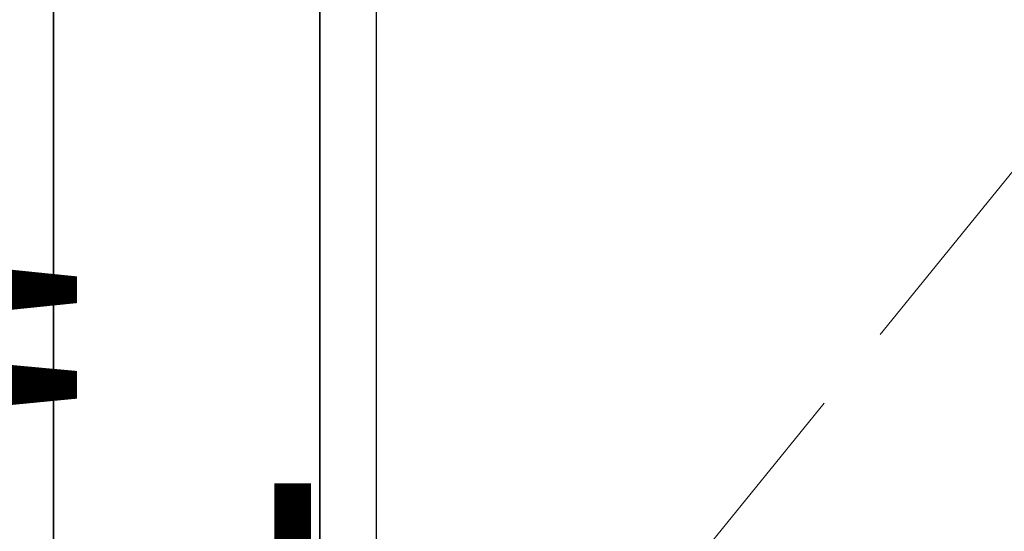
# Model space of a CAD drawing. Units: inches. Extents: x 2083 to 3317, y 1141 to 2115.
# Tile 78 of 256: x 2226 to 2259, y 1494 to 1512. Entities that reach past the tile are written whole.
import ezdxf

# ---------------------------------------------------------------- set-up
doc = ezdxf.new("R2010")
doc.units = ezdxf.units.IN
doc.linetypes.add('ACAD_ISO02W100', pattern=[15, 12, -3])
for name, color, linetype, lineweight in [('A-ANNO-DIMS', 2, 'Continuous', 18), ('A-FLOR-OPEN', 8, 'ACAD_ISO02W100', 13), ('A-WALL', 7, 'Continuous', 35)]:
    doc.layers.add(name, color=color, linetype=linetype, lineweight=lineweight)
doc.layers.add('A-WALL-PATT', color=251, linetype='Continuous', lineweight=13, true_color=0x636466)
doc.styles.get("Standard").update_dxf_attribs({"font": 'arial.ttf'})
doc.dimstyles.new('ISO-25', dxfattribs={"dimtxt": 12, "dimasz": 12, "dimexe": 1.25, "dimexo": 0.625, "dimtad": 1, "dimlunit": 3, "dimtxsty": 'Standard', "dimcen": 2.5, "dimadec": 0, "dimazin": 0, "dimtfac": 1, "dimtmove": 0, "dimatfit": 3, "dimfxl": 1, "dimarcsym": 0})

# ---------------------------------------------------------------- blocks, each defined once
blk = doc.blocks.new('*D31')
at = {"layer": 'A-ANNO-DIMS', "color": 0, "lineweight": -2, "transparency": 16777216}
for p, q in [((2237.871, 1456.649), (2237.871, 1541.915)), ((2239.393, 1444.649), (2236.621, 1444.649)), ((2237.871, 1431.548), (2237.871, 1444.649)), ((2239.393, 1431.548), (2236.621, 1431.548)), ((2237.871, 1419.548), (2237.871, 1407.548))]:
    blk.add_line(p, q, dxfattribs=at)
at = {"layer": 'A-ANNO-DIMS', "color": 0, "transparency": 16777216}
for points in [[(2235.871, 1456.649), (2239.871, 1456.649), (2237.871, 1444.649)], [(2235.871, 1419.548), (2239.871, 1419.548), (2237.871, 1431.548)]]:
    blk.add_solid(points, dxfattribs=at)
at = {"layer": 'Defpoints', "color": 0, "transparency": 16777216}
for p in [(2237.871, 1444.649), (2240.018, 1444.649), (2240.018, 1431.548)]:
    blk.add_point(p, dxfattribs=at)
at = {"layer": 'A-ANNO-DIMS', "color": 0, "transparency": 16777216, "insert": (2231.217, 1505.282), "char_height": 12, "attachment_point": 5, "rotation": 90}
blk.add_mtext('1\'-1" TYP.', dxfattribs=at)
blk = doc.blocks.new('*D45')
at = {"layer": 'A-ANNO-DIMS', "color": 0, "lineweight": -2, "transparency": 16777216}
for p, q in [((2235.96, 1478.386), (2235.96, 1531.361)), ((2418.96, 1478.386), (2418.96, 1531.361)), ((2247.96, 1530.111), (2406.96, 1530.111))]:
    blk.add_line(p, q, dxfattribs=at)
at = {"layer": 'A-ANNO-DIMS', "color": 0, "transparency": 16777216}
for points in [[(2247.96, 1532.111), (2247.96, 1528.111), (2235.96, 1530.111)], [(2406.96, 1532.111), (2406.96, 1528.111), (2418.96, 1530.111)]]:
    blk.add_solid(points, dxfattribs=at)
at = {"layer": 'Defpoints', "color": 0, "transparency": 16777216}
for p in [(2418.96, 1530.111), (2235.96, 1477.761), (2418.96, 1477.761)]:
    blk.add_point(p, dxfattribs=at)
at = {"layer": 'A-ANNO-DIMS', "color": 0, "transparency": 16777216, "insert": (2327.46, 1536.867), "char_height": 12, "attachment_point": 5}
blk.add_mtext('15\'-3"', dxfattribs=at)
blk = doc.blocks.new('*D62')
at = {"layer": 'A-ANNO-DIMS', "color": 0, "lineweight": -2, "transparency": 16777216}
for p, q in [((2235.96, 1469.386), (2235.96, 1522.361)), ((2379.96, 1469.386), (2379.96, 1522.361)), ((2247.96, 1521.111), (2367.96, 1521.111))]:
    blk.add_line(p, q, dxfattribs=at)
at = {"layer": 'A-ANNO-DIMS', "color": 0, "transparency": 16777216}
for points in [[(2247.96, 1523.111), (2247.96, 1519.111), (2235.96, 1521.111)], [(2367.96, 1523.111), (2367.96, 1519.111), (2379.96, 1521.111)]]:
    blk.add_solid(points, dxfattribs=at)
at = {"layer": 'Defpoints', "color": 0, "transparency": 16777216}
for p in [(2379.96, 1521.111), (2235.96, 1468.761), (2379.96, 1468.761)]:
    blk.add_point(p, dxfattribs=at)
at = {"layer": 'A-ANNO-DIMS', "color": 0, "transparency": 16777216, "insert": (2307.96, 1527.863), "char_height": 12, "attachment_point": 5}
blk.add_mtext('12\'-0"', dxfattribs=at)
blk = doc.blocks.new('*D64')
at = {"layer": 'A-ANNO-DIMS', "color": 0, "lineweight": -2, "transparency": 16777216}
for p, q in [((2236.585, 1702.761), (2289.56, 1702.761)), ((2288.31, 1690.761), (2288.31, 1489.761)), ((2236.585, 1477.761), (2289.56, 1477.761))]:
    blk.add_line(p, q, dxfattribs=at)
at = {"layer": 'A-ANNO-DIMS', "color": 0, "transparency": 16777216}
for points in [[(2286.31, 1690.761), (2290.31, 1690.761), (2288.31, 1702.761)], [(2286.31, 1489.761), (2290.31, 1489.761), (2288.31, 1477.761)]]:
    blk.add_solid(points, dxfattribs=at)
at = {"layer": 'Defpoints', "color": 0, "transparency": 16777216}
for p in [(2235.96, 1702.761), (2235.96, 1477.761), (2288.31, 1477.761)]:
    blk.add_point(p, dxfattribs=at)
at = {"layer": 'A-ANNO-DIMS', "color": 0, "transparency": 16777216, "insert": (2281.558, 1590.261), "char_height": 12, "attachment_point": 5, "rotation": 90}
blk.add_mtext('18\'-9"', dxfattribs=at)

msp = doc.modelspace()

# ---------------------------------------------------------------- hatches: boundary and pattern name
at = {"layer": 'A-WALL-PATT'}
h = msp.add_hatch(color=256, dxfattribs=at)
h.dxf.hatch_style = 1
h.paths.add_polyline_path([(3126.96, 2020.761), (2748.96, 2020.761), (2604.96, 2020.761), (2226.96, 2020.761), (2226.96, 1702.761), (2466.96, 1702.761), (2466.96, 1582.761), (2418.96, 1582.761), (2418.96, 1477.761), (2226.96, 1477.761), (2226.96, 1263.261), (2544.96, 1263.261), (2544.96, 1411.761), (2604.96, 1411.761), (2685.96, 1411.761), (2685.96, 1420.761), (2604.96, 1420.761), (2604.96, 1573.761), (2604.96, 1702.761), (2604.96, 2011.761), (2748.96, 2011.761), (2748.96, 1702.761), (2862.96, 1702.761), (2862.96, 1621.761), (2871.96, 1621.761), (2871.96, 1702.761), (2883.96, 1702.761), (2883.96, 1706.939, -0.026459), (2883.96, 1711.761), (2757.96, 1711.761), (2757.96, 1807.761), (2787.96, 1807.761), (2787.96, 1812.261), (2757.96, 1812.261), (2757.96, 2011.761), (2877.96, 2011.761), (2877.96, 1812.261), (2847.96, 1812.261), (2847.96, 1807.761), (2889.836, 1807.761), (2889.836, 1812.261), (2882.46, 1812.261), (2882.46, 2011.761), (3117.96, 2011.761), (3117.96, 1812.261), (2937.836, 1812.261), (2937.836, 1807.761), (2995.71, 1807.761), (2995.71, 1796.118), (3000.21, 1796.118), (3000.21, 1807.761), (3117.96, 1807.761), (3117.96, 1711.761), (3000.21, 1711.761), (3000.21, 1760.118), (2998.573, 1760.118, -0.020711), (2995.71, 1760.118), (2995.71, 1711.761), (2931.96, 1711.761), (2931.96, 1702.761), (3126.96, 1702.761)])
h.paths.add_polyline_path([(2471.46, 2011.761), (2471.46, 1810.011), (2462.717, 1810.011), (2462.717, 1805.511), (2505.96, 1805.511), (2505.96, 1810.011), (2475.96, 1810.011), (2475.96, 2011.761), (2595.96, 2011.761), (2595.96, 1810.011), (2565.96, 1810.011), (2565.96, 1805.511), (2595.96, 1805.511), (2595.96, 1711.761), (2235.96, 1711.761), (2235.96, 1805.511), (2353.71, 1805.511), (2353.71, 1796.054), (2358.21, 1796.054), (2358.21, 1805.511), (2414.717, 1805.511), (2414.717, 1810.011), (2235.96, 1810.011), (2235.96, 2011.761)], flags=16)
h.paths.add_polyline_path([(2270.205, 1994.61), (2270.205, 1970.61), (2246.205, 1970.61), (2246.205, 1994.61)], flags=0)
edge = h.paths.add_edge_path(flags=0)
edge.add_ellipse((2332.027, 1899.798), major_axis=(-3.043, 3.043), ratio=0.168252, start_angle=-161.3322, end_angle=-156.3071, ccw=False)
edge.add_ellipse((2333.082, 1898.744), major_axis=(-1.055, 1.055), ratio=0.453532, start_angle=-123.371, end_angle=-94.1591)
edge = h.paths.add_edge_path(flags=0)
edge.add_ellipse((2332.027, 1968.876), major_axis=(3.043, 3.043), ratio=0.168252, start_angle=18.6678, end_angle=23.6929)
edge.add_spline(control_points=[(2332.926, 1970.691), (2332.227, 1970.336), (2330.894, 1969.659), (2328.413, 1970.932), (2327.204, 1967.749), (2324.71, 1969.956), (2322.533, 1967.012), (2320.013, 1971.296), (2317.68, 1968.158), (2316.041, 1967.102), (2315.427, 1966.81)], knot_values=[0, 0, 0, 0, 2.267059, 4.324559, 6.685584, 8.878641, 11.121502, 14.300359, 17.755284, 19.732645, 19.732645, 19.732645, 19.732645], degree=3, periodic=0)
edge.add_ellipse((2332.027, 1968.876), major_axis=(3.043, 3.043), ratio=0.168252, start_angle=18.6678, end_angle=23.6929, ccw=False)
edge.add_ellipse((2333.082, 1969.931), major_axis=(1.055, 1.055), ratio=0.453532, start_angle=56.629, end_angle=85.8409, ccw=False)
edge = h.paths.add_edge_path(flags=0)
edge.add_spline(control_points=[(2296.428, 1967.988), (2293.628, 1965.336), (2287.704, 1959.727), (2299.744, 1949.996), (2294.533, 1935.669), (2290.573, 1920.604), (2293.394, 1909.974), (2296.185, 1904.967)], knot_values=[0.099185, 0.099185, 0.099185, 0.099185, 0.345301, 0.619822, 0.982653, 1.386093, 1.810555, 1.810555, 1.810555, 1.810555], degree=3, periodic=0)
edge.add_spline(control_points=[(2296.185, 1904.967), (2297.384, 1902.619), (2298.001, 1901.949), (2298.553, 1901.468)], knot_values=[0.006246, 0.006246, 0.006246, 0.006246, 0.055476, 0.055476, 0.055476, 0.055476], degree=3, periodic=0)
edge.add_spline(control_points=[(2298.553, 1901.468), (2297.259, 1900.923), (2295.225, 1900.232), (2293.06, 1900.614), (2292.101, 1900.788), (2292.09, 1900.791)], knot_values=[0.312835, 0.312835, 0.312835, 0.312835, 0.40178, 0.474987, 0.475903, 0.475903, 0.475903, 0.475903], degree=3, periodic=0)
edge.add_arc((2292.794, 1904.664), 3.937, 215.4209, 259.6982, ccw=False)
edge.add_spline(control_points=[(2289.585, 1902.382), (2289.477, 1902.535), (2289.368, 1902.688), (2289.261, 1902.841)], knot_values=[0.102872, 0.102872, 0.102872, 0.102872, 0.116896, 0.116896, 0.116896, 0.116896], degree=3, periodic=0)
edge.add_spline(control_points=[(2289.261, 1902.841), (2288.687, 1902.55), (2287.64, 1902.02), (2285.881, 1901.874), (2283.853, 1901.504), (2281.72, 1899.711), (2278.467, 1899.493), (2276.157, 1901.883), (2272.259, 1899.804), (2267.778, 1901.843), (2262.244, 1900.184), (2257.415, 1901.782), (2254.318, 1900.726), (2253.178, 1900.337)], knot_values=[0, 0, 0, 0, 1.907977, 3.477176, 5.261074, 7.972851, 11.680248, 13.717921, 16.939592, 22.789562, 27.502503, 33.595215, 37.145618, 37.145618, 37.145618, 37.145618], degree=3, periodic=0)
edge.add_line((2253.178, 1900.337), (2250.244, 1902.841))
edge.add_line((2250.244, 1902.841), (2250.244, 1965.833))
edge.add_line((2250.244, 1965.833), (2253.178, 1968.337))
edge.add_spline(control_points=[(2253.178, 1968.337), (2254.318, 1967.948), (2257.415, 1966.892), (2262.244, 1968.49), (2267.778, 1966.831), (2271.527, 1968.537), (2273.876, 1967.828), (2274.207, 1967.728)], knot_values=[0, 0, 0, 0, 0.09018, 0.244935, 0.364644, 0.513233, 0.537855, 0.537855, 0.537855, 0.537855], degree=3, periodic=0)
edge.add_arc((2274.353, 1963.793), 3.937, 72.0511, 92.1279, ccw=False)
edge.add_arc((2281.297, 1985.23), 18.596, 252.0511, 288.5657)
edge.add_arc((2292.317, 1956.029), 12.646, 71.0268, 113.7782, ccw=False)
edge = h.paths.add_edge_path(flags=0)
edge.add_spline(control_points=[(2274.899, 1951.856), (2275.066, 1951.617), (2275.233, 1951.377), (2275.398, 1951.136)], knot_values=[1.409916, 1.409916, 1.409916, 1.409916, 1.43159, 1.43159, 1.43159, 1.43159], degree=3, periodic=0)
edge.add_spline(control_points=[(2275.398, 1951.136), (2275.792, 1950.562), (2276.179, 1949.984), (2276.546, 1949.397)], knot_values=[1.358238, 1.358238, 1.358238, 1.358238, 1.409916, 1.409916, 1.409916, 1.409916], degree=3, periodic=0)
edge.add_line((2276.546, 1949.397), (2277.437, 1947.862))
edge.add_spline(control_points=[(2277.437, 1947.862), (2276.304, 1945.673), (2274.64, 1942.427), (2274.632, 1938.094), (2272.799, 1930.852), (2274.356, 1943.897), (2275.948, 1947.923), (2276.546, 1949.397)], knot_values=[0.005632, 0.005632, 0.005632, 0.005632, 0.186014, 0.266002, 0.357087, 0.59639, 0.739732, 0.739732, 0.739732, 0.739732], degree=3, periodic=0)
edge.add_spline(control_points=[(2276.546, 1949.397), (2276.179, 1949.984), (2275.792, 1950.562), (2275.398, 1951.136)], knot_values=[1.358238, 1.358238, 1.358238, 1.358238, 1.409916, 1.409916, 1.409916, 1.409916], degree=3, periodic=0)
edge.add_spline(control_points=[(2275.398, 1951.136), (2274.943, 1950.08), (2274.208, 1948.025), (2273.935, 1944.851), (2272.469, 1937.627), (2273.466, 1945.696), (2274.701, 1951.059), (2274.899, 1951.856)], knot_values=[0.104364, 0.104364, 0.104364, 0.104364, 0.189636, 0.269624, 0.36071, 0.600013, 0.644622, 0.644622, 0.644622, 0.644622], degree=3, periodic=0)
h.paths.add_polyline_path([(2269.168, 1963.128, -0.357527), (2268.171, 1960.976, -0.092561), (2268.171, 1939.436, -0.357527), (2269.168, 1937.285, -0.357527), (2267.016, 1938.282, -0.164785), (2254.686, 1938.282, -0.357527), (2252.534, 1937.285, -0.357527), (2253.531, 1939.436, -0.092561), (2253.531, 1960.976, -0.357527), (2252.534, 1963.128, -0.357527), (2254.686, 1962.131, -0.164785), (2267.016, 1962.131, -0.357527)], flags=0)
h.paths.add_polyline_path([(2248.874, 1967.802), (2248.874, 1957.028), (2249.458, 1957.028), (2249.458, 1911.647), (2248.874, 1911.647), (2248.874, 1900.873), (2246.512, 1900.873, 0.197327), (2244.15, 1902.457), (2244.15, 1966.218, 0.197327), (2246.512, 1967.802)], flags=0)
h.paths.add_polyline_path([(2269.168, 1931.389, -0.357527), (2268.171, 1929.238, -0.092561), (2268.171, 1907.698, -0.357527), (2269.168, 1905.547, -0.357527), (2267.016, 1906.544, -0.164785), (2254.686, 1906.544, -0.357527), (2252.534, 1905.547, -0.357527), (2253.531, 1907.698, -0.092561), (2253.531, 1929.238, -0.357527), (2252.534, 1931.389, -0.357527), (2254.686, 1930.392, -0.164785), (2267.016, 1930.392, -0.357527)], flags=0)
edge = h.paths.add_edge_path(flags=0)
edge.add_spline(control_points=[(2276.197, 1906.724), (2276.168, 1909.029), (2276.114, 1913.372), (2270.598, 1924.925), (2273.905, 1919.013), (2275.922, 1916.262), (2275.475, 1912.402), (2277.258, 1910.381), (2276.696, 1908.225), (2276.646, 1906.813), (2276.618, 1906.008)], knot_values=[0, 0, 0, 0, 8.61026, 16.221274, 18.843057, 23.804898, 27.440828, 29.356102, 31.203478, 33.650687, 33.650687, 33.650687, 33.650687], degree=3, periodic=0)
edge.add_spline(control_points=[(2276.618, 1906.008), (2276.623, 1905.624), (2276.498, 1904.629), (2275.442, 1903.855), (2274.937, 1903.08), (2274.859, 1902.841)], knot_values=[0.156488, 0.156488, 0.156488, 0.156488, 0.184398, 0.231376, 0.250598, 0.250598, 0.250598, 0.250598], degree=3, periodic=0)
edge.add_line((2274.859, 1902.841), (2276.506, 1902.841))
edge.add_spline(control_points=[(2276.506, 1902.841), (2276.788, 1903.085), (2277.665, 1904.125), (2278.25, 1904.341), (2277.654, 1908.527), (2278.156, 1906.228), (2278.1, 1905.286), (2278.847, 1904.069), (2277.857, 1903.415), (2277.874, 1902.991), (2277.904, 1902.841)], knot_values=[0.059574, 0.059574, 0.059574, 0.059574, 0.080753, 0.103741, 0.16972, 0.176036, 0.207137, 0.240474, 0.262341, 0.27366, 0.27366, 0.27366, 0.27366], degree=3, periodic=0)
edge.add_line((2277.904, 1902.841), (2280.03, 1902.841))
edge.add_spline(control_points=[(2280.03, 1902.841), (2279.888, 1903.088), (2279.499, 1903.982), (2280.152, 1905.939), (2278.104, 1909.658), (2279.762, 1907.185), (2280.328, 1904.875), (2280.485, 1903.49), (2281.463, 1903.249), (2281.758, 1902.936), (2281.834, 1902.841)], knot_values=[0.013856, 0.013856, 0.013856, 0.013856, 0.034874, 0.088867, 0.107879, 0.126738, 0.158714, 0.193757, 0.217487, 0.226722, 0.226722, 0.226722, 0.226722], degree=3, periodic=0)
edge.add_spline(control_points=[(2281.834, 1902.841), (2281.788, 1902.827), (2281.647, 1902.783), (2281.396, 1902.859), (2281.088, 1902.985), (2280.721, 1903.061), (2280.333, 1903.026), (2280.125, 1902.899), (2280.03, 1902.841)], knot_values=[0, 0, 0, 0, 0.14413, 0.435517, 0.749276, 1.153046, 1.548371, 1.878348, 1.878348, 1.878348, 1.878348], degree=3, periodic=0)
edge.add_line((2280.03, 1902.841), (2277.904, 1902.841))
edge.add_spline(control_points=[(2277.904, 1902.841), (2277.893, 1902.796), (2277.865, 1902.68), (2277.607, 1902.687), (2277.274, 1902.801), (2276.838, 1902.62), (2276.584, 1902.789), (2276.506, 1902.841)], knot_values=[0, 0, 0, 0, 0.127189, 0.326199, 0.628009, 1.24357, 1.515331, 1.515331, 1.515331, 1.515331], degree=3, periodic=0)
edge.add_line((2276.506, 1902.841), (2274.859, 1902.841))
edge.add_spline(control_points=[(2274.859, 1902.841), (2274.814, 1902.899), (2274.725, 1903.013), (2274.493, 1903.119), (2274.244, 1902.961), (2273.937, 1903.185), (2273.614, 1902.983), (2273.408, 1902.883), (2273.322, 1902.841)], knot_values=[0, 0, 0, 0, 0.21843, 0.436957, 0.687977, 0.990379, 1.398396, 1.69185, 1.69185, 1.69185, 1.69185], degree=3, periodic=0)
edge.add_spline(control_points=[(2273.322, 1902.841), (2273.617, 1903.446), (2274.274, 1904.538), (2276.027, 1904.574), (2276.207, 1906.584), (2276.197, 1906.724)], knot_values=[0.012227, 0.012227, 0.012227, 0.012227, 0.059472, 0.106218, 0.134458, 0.134458, 0.134458, 0.134458], degree=3, periodic=0)
h.paths.add_polyline_path([(2270.776, 1897.79), (2270.776, 1873.79), (2246.776, 1873.79), (2246.776, 1897.79)], flags=0)
h.paths.add_polyline_path([(2353.71, 1760.005), (2353.71, 1760.054), (2358.21, 1760.054, -0.033729)], flags=0)
h.paths.add_polyline_path([(2321.819, 1737.529), (2341.995, 1737.529, -0.414214), (2343.203, 1736.321), (2343.203, 1721.021, -0.414214), (2341.995, 1719.813), (2321.819, 1719.813, -0.414214), (2320.611, 1721.021), (2320.611, 1736.321, -0.414214)], flags=0)
h.paths.add_polyline_path([(2324.235, 1736.321), (2339.579, 1736.321, -0.414214), (2341.995, 1733.905), (2341.995, 1725.45, -0.414214), (2339.579, 1723.034), (2333.681, 1723.034), (2333.845, 1722.045, -0.870646), (2335.425, 1721.826, -0.767327), (2333.923, 1721.423), (2331.291, 1721.423, -0.767327), (2329.788, 1721.826, -0.870646), (2331.368, 1722.045), (2331.533, 1723.034), (2324.235, 1723.034, -0.414214), (2321.819, 1725.45), (2321.819, 1733.905, -0.414214)], flags=0)
h.paths.add_polyline_path([(2570.484, 1928.615), (2589.684, 1928.615), (2590.169, 1928.615), (2590.169, 1904.993), (2570.484, 1904.993)], flags=0)
h.paths.add_polyline_path([(2574.447, 1927.264, -1), (2572.829, 1927.264, -1)], flags=0)
h.paths.add_polyline_path([(2573.09, 1926.941), (2573.925, 1927.776), (2574.148, 1927.553), (2573.313, 1926.718)], flags=0)
h.paths.add_polyline_path([(2578.779, 1919.73, -1), (2571.592, 1919.73, -1)], flags=0)
h.paths.add_polyline_path([(2578.385, 1919.73, -1), (2571.985, 1919.73, -1)], flags=0)
h.paths.add_polyline_path([(2331.596, 1729.476, -1), (2333.618, 1729.476, -1)], flags=0)
h.paths.add_polyline_path([(2578.034, 1927.264, -1), (2576.416, 1927.264, -1)], flags=0)
h.paths.add_polyline_path([(2576.689, 1927.531), (2576.912, 1927.754), (2577.747, 1926.919), (2577.524, 1926.696)], flags=0)
h.paths.add_polyline_path([(2578.139, 1909.86, -1), (2572.232, 1909.86, -1)], flags=0)
h.paths.add_polyline_path([(2577.745, 1909.86, -1), (2572.625, 1909.86, -1)], flags=0)
h.paths.add_polyline_path([(2583.798, 1927.264, -1), (2582.179, 1927.264, -1)], flags=0)
h.paths.add_polyline_path([(2582.719, 1927.754), (2583.554, 1926.919), (2583.331, 1926.696), (2582.496, 1927.531)], flags=0)
h.paths.add_polyline_path([(2582.496, 1927.531), (2582.719, 1927.754), (2583.554, 1926.919), (2583.331, 1926.696)], flags=0)
h.paths.add_polyline_path([(2587.739, 1920.53, -1), (2581.832, 1920.53, -1)], flags=0)
h.paths.add_polyline_path([(2587.345, 1920.53, -1), (2582.225, 1920.53, -1)], flags=0)
h.paths.add_polyline_path([(2587.385, 1927.264, -1), (2585.766, 1927.264, -1)], flags=0)
h.paths.add_polyline_path([(2586.082, 1926.98), (2586.917, 1927.815), (2587.14, 1927.593), (2586.305, 1926.758)], flags=0)
h.paths.add_polyline_path([(2588.379, 1910.66, -1), (2581.192, 1910.66, -1)], flags=0)
h.paths.add_polyline_path([(2587.985, 1910.66, -1), (2581.585, 1910.66, -1)], flags=0)
h.paths.add_polyline_path([(2417.168, 1729.478), (2437.344, 1729.478, -0.414214), (2438.552, 1728.27), (2438.552, 1712.969, -0.414214), (2437.344, 1711.761), (2417.168, 1711.761, -0.414214), (2415.96, 1712.969), (2415.96, 1728.27, -0.414214)], flags=0)
h.paths.add_polyline_path([(2419.584, 1728.27), (2434.928, 1728.27, -0.414214), (2437.344, 1725.854), (2437.344, 1717.398, -0.414214), (2434.928, 1714.983), (2429.029, 1714.983), (2429.194, 1713.994, -0.870646), (2430.774, 1713.775, -0.767327), (2429.271, 1713.372), (2426.64, 1713.372, -0.767327), (2425.137, 1713.775, -0.870646), (2426.717, 1713.994), (2426.882, 1714.983), (2419.584, 1714.983, -0.414214), (2417.168, 1717.398), (2417.168, 1725.854, -0.414214)], flags=0)
h.paths.add_polyline_path([(2419.584, 1728.27), (2434.928, 1728.27, -0.414214), (2437.344, 1725.854), (2437.344, 1717.398, -0.414214), (2434.928, 1714.983), (2429.029, 1714.983), (2428.358, 1719.009), (2427.553, 1719.009), (2426.882, 1714.983), (2419.584, 1714.983, -0.414214), (2417.168, 1717.398), (2417.168, 1725.854, -0.414214)], flags=0)
h.paths.add_polyline_path([(2426.944, 1721.425, -1), (2428.967, 1721.425, -1)], flags=0)
h.paths.add_polyline_path([(2475.96, 1702.761), (2595.96, 1702.761), (2595.96, 1582.761), (2475.96, 1582.761)], flags=16)
h.paths.add_polyline_path([(2427.96, 1573.761), (2595.96, 1573.761), (2595.96, 1468.761), (2595.96, 1420.761), (2384.46, 1420.761), (2384.46, 1468.761), (2427.96, 1468.761)], flags=16)
h.paths.add_polyline_path([(2379.96, 1468.761), (2379.96, 1420.761), (2235.96, 1420.761), (2235.96, 1468.761)], flags=16)
h.paths.add_polyline_path([(2317.816, 1466.696), (2337.992, 1466.696, -0.414214), (2339.2, 1465.488), (2339.2, 1450.187, -0.414214), (2337.992, 1448.979), (2317.816, 1448.979, -0.414214), (2316.608, 1450.187), (2316.608, 1465.488, -0.414214)], flags=0)
h.paths.add_polyline_path([(2320.232, 1465.488), (2335.576, 1465.488, -0.414214), (2337.992, 1463.072), (2337.992, 1454.616, -0.414214), (2335.576, 1452.2), (2329.677, 1452.2), (2329.842, 1451.212, -0.870646), (2331.422, 1450.992, -0.767327), (2329.92, 1450.59), (2327.288, 1450.59, -0.767327), (2325.785, 1450.992, -0.870646), (2327.365, 1451.212), (2327.53, 1452.2), (2320.232, 1452.2, -0.414214), (2317.816, 1454.616), (2317.816, 1463.072, -0.414214)], flags=0)
h.paths.add_polyline_path([(2320.232, 1465.488), (2335.576, 1465.488, -0.414214), (2337.992, 1463.072), (2337.992, 1454.616, -0.414214), (2335.576, 1452.2), (2329.677, 1452.2), (2329.006, 1456.227), (2328.201, 1456.227), (2327.53, 1452.2), (2320.232, 1452.2, -0.414214), (2317.816, 1454.616), (2317.816, 1463.072, -0.414214)], flags=0)
h.paths.add_polyline_path([(2327.593, 1458.643, -1), (2329.615, 1458.643, -1)], flags=0)
h.paths.add_polyline_path([(2244.412, 1433.34), (2241.921, 1433.34, -0.414214), (2240.018, 1435.244), (2240.018, 1440.953, -0.414211), (2241.921, 1442.856), (2244.412, 1442.856, -1.976472)], flags=0)
h.paths.add_polyline_path([(2245.357, 1434.398, -0.414214), (2245.357, 1441.799, -2.144098)], flags=0)
h.paths.add_polyline_path([(2535.96, 1416.261), (2535.96, 1272.261), (2235.96, 1272.261), (2235.96, 1416.261)], flags=16)
h.paths.add_polyline_path([(2260.12, 1384.293), (2260.12, 1362.039), (2237.865, 1362.039), (2237.865, 1384.293)], flags=0)
edge = h.paths.add_edge_path(flags=0)
edge.add_line((2318.252, 1362.093), (2318.146, 1362.001))
edge.add_ellipse((2317.445, 1360.431), major_axis=(2.822, 2.822), ratio=0.168252, start_angle=18.6678, end_angle=20.9481, ccw=False)
edge.add_ellipse((2318.423, 1361.409), major_axis=(0.978, 0.978), ratio=0.453532, start_angle=56.629, end_angle=70.2262, ccw=False)
edge = h.paths.add_edge_path(flags=0)
edge.add_line((2319.107, 1295.571), (2319.015, 1295.677))
edge.add_ellipse((2317.445, 1296.378), major_axis=(-2.822, 2.822), ratio=0.168252, start_angle=-161.3322, end_angle=-159.0519, ccw=False)
edge.add_ellipse((2318.423, 1295.4), major_axis=(-0.978, 0.978), ratio=0.453532, start_angle=-123.371, end_angle=-109.7738)
edge = h.paths.add_edge_path(flags=0)
edge.add_spline(control_points=[(2284.21, 1301.17), (2284.581, 1300.445), (2284.891, 1299.892), (2285.16, 1299.461)], knot_values=[0.039066, 0.039066, 0.039066, 0.039066, 0.055476, 0.055476, 0.055476, 0.055476], degree=3, periodic=0)
edge.add_line((2285.16, 1299.461), (2284.21, 1301.17))
edge = h.paths.add_edge_path(flags=0)
edge.add_line((2280.412, 1297.298), (2283.37, 1297.036))
edge.add_line((2283.37, 1297.036), (2286.406, 1297.926))
edge.add_spline(control_points=[(2286.406, 1297.926), (2285.305, 1297.463), (2284.345, 1297.129), (2283.37, 1297.036)], knot_values=[0.394369, 0.394369, 0.394369, 0.394369, 0.475903, 0.475903, 0.475903, 0.475903], degree=3, periodic=0)
edge.add_spline(control_points=[(2283.37, 1297.036), (2283.281, 1297.028), (2282.316, 1296.957), (2281.313, 1297.134), (2280.423, 1297.296), (2280.412, 1297.298)], knot_values=[0.312835, 0.312835, 0.312835, 0.312835, 0.320246, 0.393453, 0.394369, 0.394369, 0.394369, 0.394369], degree=3, periodic=0)
edge = h.paths.add_edge_path(flags=0)
edge.add_line((2284.436, 1359.607), (2280.446, 1355.328))
edge.add_line((2280.446, 1355.328), (2279.58, 1351.018))
edge.add_line((2279.58, 1351.018), (2282.413, 1346.58))
edge.add_spline(control_points=[(2282.413, 1346.58), (2283.153, 1345.589), (2284.253, 1344.029), (2284.801, 1342.387), (2284.935, 1341.806)], knot_values=[1.240098, 1.240098, 1.240098, 1.240098, 1.332892, 1.382712, 1.382712, 1.382712, 1.382712], degree=3, periodic=0)
edge.add_spline(control_points=[(2284.935, 1341.806), (2285.319, 1340.141), (2285.233, 1338.409), (2284.91, 1336.654)], knot_values=[1.097484, 1.097484, 1.097484, 1.097484, 1.240098, 1.240098, 1.240098, 1.240098], degree=3, periodic=0)
edge.add_spline(control_points=[(2284.91, 1336.654), (2284.587, 1334.899), (2284.027, 1333.12), (2283.463, 1331.361)], knot_values=[0.95487, 0.95487, 0.95487, 0.95487, 1.097484, 1.097484, 1.097484, 1.097484], degree=3, periodic=0)
edge.add_line((2283.463, 1331.361), (2281.89, 1326.153))
edge.add_line((2281.89, 1326.153), (2280.756, 1321.056))
edge.add_line((2280.756, 1321.056), (2280.299, 1316.002))
edge.add_line((2280.299, 1316.002), (2280.716, 1310.95))
edge.add_line((2280.716, 1310.95), (2282.028, 1305.972))
edge.add_line((2282.028, 1305.972), (2284.21, 1301.17))
edge.add_spline(control_points=[(2284.21, 1301.17), (2283.341, 1302.73), (2282.612, 1304.336), (2282.028, 1305.972)], knot_values=[0.099185, 0.099185, 0.099185, 0.099185, 0.241799, 0.241799, 0.241799, 0.241799], degree=3, periodic=0)
edge.add_spline(control_points=[(2282.028, 1305.972), (2281.444, 1307.608), (2281.005, 1309.273), (2280.716, 1310.95)], knot_values=[0.241799, 0.241799, 0.241799, 0.241799, 0.384413, 0.384413, 0.384413, 0.384413], degree=3, periodic=0)
edge.add_spline(control_points=[(2280.716, 1310.95), (2280.433, 1312.588), (2280.289, 1314.277), (2280.299, 1315.962), (2280.299, 1316.002)], knot_values=[0.384413, 0.384413, 0.384413, 0.384413, 0.523647, 0.527028, 0.527028, 0.527028, 0.527028], degree=3, periodic=0)
edge.add_spline(control_points=[(2280.299, 1316.002), (2280.312, 1317.687), (2280.478, 1319.368), (2280.756, 1321.056)], knot_values=[0.527028, 0.527028, 0.527028, 0.527028, 0.669642, 0.669642, 0.669642, 0.669642], degree=3, periodic=0)
edge.add_spline(control_points=[(2280.756, 1321.056), (2281.035, 1322.744), (2281.426, 1324.44), (2281.89, 1326.153)], knot_values=[0.669642, 0.669642, 0.669642, 0.669642, 0.812256, 0.812256, 0.812256, 0.812256], degree=3, periodic=0)
edge.add_spline(control_points=[(2281.89, 1326.153), (2282.264, 1327.533), (2282.788, 1329.262), (2283.353, 1331.018), (2283.463, 1331.361)], knot_values=[0.812256, 0.812256, 0.812256, 0.812256, 0.927087, 0.95487, 0.95487, 0.95487, 0.95487], degree=3, periodic=0)
edge.add_line((2283.463, 1331.361), (2284.91, 1336.654))
edge.add_line((2284.91, 1336.654), (2284.935, 1341.806))
edge.add_line((2284.935, 1341.806), (2282.413, 1346.58))
edge.add_spline(control_points=[(2282.413, 1346.58), (2281.275, 1348.104), (2280.078, 1349.57), (2279.58, 1351.018)], knot_values=[1.382712, 1.382712, 1.382712, 1.382712, 1.525326, 1.525326, 1.525326, 1.525326], degree=3, periodic=0)
edge.add_spline(control_points=[(2279.58, 1351.018), (2279.443, 1351.415), (2279.136, 1352.857), (2279.735, 1354.29), (2280.446, 1355.328)], knot_values=[1.525326, 1.525326, 1.525326, 1.525326, 1.564439, 1.667941, 1.667941, 1.667941, 1.667941], degree=3, periodic=0)
edge.add_spline(control_points=[(2280.446, 1355.328), (2281.426, 1356.758), (2282.931, 1358.183), (2284.436, 1359.607)], knot_values=[1.667941, 1.667941, 1.667941, 1.667941, 1.810555, 1.810555, 1.810555, 1.810555], degree=3, periodic=0)
edge.add_arc((2280.623, 1348.518), 11.726, 71.0268, 113.7782)
edge.add_arc((2270.405, 1375.595), 17.244, 252.0511, 288.5657, ccw=False)
edge.add_arc((2263.966, 1355.718), 3.651, 72.0511, 92.1279)
edge.add_arc((2263.966, 1355.718), 3.651, 92.1279, 177.9851)
edge.add_spline(control_points=[(2260.318, 1355.846), (2260.26, 1354.221), (2260.551, 1350.187), (2262.999, 1346.766), (2264.473, 1344.649)], knot_values=[1.43159, 1.43159, 1.43159, 1.43159, 1.564144, 1.770695, 1.770695, 1.770695, 1.770695], degree=3, periodic=0)
edge.add_line((2264.473, 1344.649), (2264.936, 1343.983))
edge.add_spline(control_points=[(2263.801, 1340.248), (2263.843, 1340.514), (2264.067, 1341.756), (2264.513, 1343.002), (2264.935, 1343.981)], knot_values=[0.53657, 0.53657, 0.53657, 0.53657, 0.559349, 0.644622, 0.644622, 0.644622, 0.644622], degree=3, periodic=0)
edge.add_spline(control_points=[(2264.935, 1343.981), (2265.118, 1343.715), (2265.299, 1343.448), (2265.477, 1343.179)], knot_values=[1.384077, 1.384077, 1.384077, 1.384077, 1.409916, 1.409916, 1.409916, 1.409916], degree=3, periodic=0)
edge.add_spline(control_points=[(2265.477, 1343.179), (2265.655, 1342.911), (2265.829, 1342.641), (2265.999, 1342.369)], knot_values=[1.358238, 1.358238, 1.358238, 1.358238, 1.384077, 1.384077, 1.384077, 1.384077], degree=3, periodic=0)
edge.add_line((2265.999, 1342.369), (2266.826, 1340.946))
edge.add_spline(control_points=[(2266.826, 1340.946), (2268.894, 1337.09), (2271.398, 1325.843), (2270.516, 1310.569), (2275.919, 1301.861), (2277.79, 1299.199)], knot_values=[0.116896, 0.116896, 0.116896, 0.116896, 0.472987, 1.050969, 1.313793, 1.313793, 1.313793, 1.313793], degree=3, periodic=0)
edge.add_spline(control_points=[(2277.79, 1299.199), (2277.839, 1299.128), (2277.889, 1299.057), (2277.94, 1298.987)], knot_values=[0.109884, 0.109884, 0.109884, 0.109884, 0.116896, 0.116896, 0.116896, 0.116896], degree=3, periodic=0)
edge.add_line((2277.94, 1298.987), (2277.789, 1299.199))
edge.add_spline(control_points=[(2277.789, 1299.199), (2277.257, 1298.929), (2276.286, 1298.438), (2275.039, 1298.334), (2274.383, 1298.239), (2274.215, 1298.209)], knot_values=[33.12187, 33.12187, 33.12187, 33.12187, 35.029056, 36.598255, 37.144827, 37.144827, 37.144827, 37.144827], degree=3, periodic=0)
edge.add_line((2274.215, 1298.209), (2273.073, 1297.893))
edge.add_spline(control_points=[(2273.073, 1297.893), (2272.323, 1297.58), (2271.039, 1296.511), (2269.248, 1296.226), (2268.423, 1296.375)], knot_values=[26.532584, 26.532584, 26.532584, 26.532584, 29.198919, 31.839101, 31.839101, 31.839101, 31.839101], degree=3, periodic=0)
edge.add_line((2268.423, 1296.375), (2263.879, 1297.458))
edge.add_spline(control_points=[(2263.879, 1297.458), (2263.556, 1297.359), (2261.86, 1296.839), (2260.239, 1297.282), (2258.933, 1297.516)], knot_values=[15.919551, 15.919551, 15.919551, 15.919551, 16.939592, 21.226067, 21.226067, 21.226067, 21.226067], degree=3, periodic=0)
edge.add_line((2258.933, 1297.516), (2254.055, 1297.329))
edge.add_spline(control_points=[(2254.055, 1297.329), (2253.756, 1297.296), (2252.114, 1297.165), (2250.462, 1297.544), (2249.13, 1297.668)], knot_values=[5.306517, 5.306517, 5.306517, 5.306517, 6.276435, 10.613034, 10.613034, 10.613034, 10.613034], degree=3, periodic=0)
edge.add_line((2249.13, 1297.668), (2244.332, 1296.878))
edge.add_line((2244.332, 1296.878), (2241.611, 1299.199))
edge.add_line((2241.611, 1299.199), (2241.611, 1357.609))
edge.add_line((2241.611, 1357.609), (2244.332, 1359.931))
edge.add_line((2244.332, 1359.931), (2252.729, 1359.543))
edge.add_spline(control_points=[(2252.729, 1359.543), (2252.871, 1359.546), (2253.306, 1359.548), (2253.74, 1359.514), (2254.032, 1359.482)], knot_values=[0.233291, 0.233291, 0.233291, 0.233291, 0.244935, 0.268927, 0.268927, 0.268927, 0.268927], degree=3, periodic=0)
edge.add_line((2254.032, 1359.482), (2259.587, 1359.416))
edge.add_spline(control_points=[(2259.587, 1359.416), (2260.677, 1359.629), (2262.073, 1359.897), (2263.524, 1359.459), (2263.83, 1359.366)], knot_values=[0.422516, 0.422516, 0.422516, 0.422516, 0.513233, 0.537855, 0.537855, 0.537855, 0.537855], degree=3, periodic=0)
edge.add_arc((2263.966, 1355.718), 3.651, 72.0511, 92.1279, ccw=False)
edge.add_arc((2270.405, 1375.595), 17.244, 252.0511, 288.5657)
edge.add_arc((2280.623, 1348.518), 11.726, 71.0268, 113.7782, ccw=False)
h.paths.add_polyline_path([(2240.341, 1359.435), (2240.341, 1349.444), (2240.882, 1349.444), (2240.882, 1307.365), (2240.341, 1307.365), (2240.341, 1297.374), (2238.15, 1297.374, 0.197327), (2235.96, 1298.843), (2235.96, 1357.966, 0.197327), (2238.15, 1359.435)], flags=0)
h.paths.add_polyline_path([(2259.158, 1355.101, -0.357527), (2258.233, 1353.106, -0.092561), (2258.233, 1333.133, -0.357527), (2259.158, 1331.138, -0.357527), (2257.163, 1332.062, -0.164785), (2245.729, 1332.062, -0.357527), (2243.735, 1331.138, -0.357527), (2244.659, 1333.133, -0.092561), (2244.659, 1353.106, -0.357527), (2243.735, 1355.101, -0.357527), (2245.729, 1354.176, -0.164785), (2257.163, 1354.176, -0.357527)], flags=0)
edge = h.paths.add_edge_path(flags=0)
edge.add_line((2265.999, 1342.369), (2266.826, 1340.946))
edge.add_line((2266.826, 1340.946), (2265.308, 1337.814))
edge.add_line((2265.308, 1337.814), (2264.358, 1334.653))
edge.add_line((2264.358, 1334.653), (2264.262, 1333.8))
edge.add_spline(control_points=[(2264.262, 1333.8), (2264.208, 1333.187), (2264.162, 1332.366), (2264.007, 1331.414), (2263.969, 1331.202)], knot_values=[0.464444, 0.464444, 0.464444, 0.464444, 0.516691, 0.531608, 0.531608, 0.531608, 0.531608], degree=3, periodic=0)
edge.add_spline(control_points=[(2263.969, 1331.202), (2263.775, 1330.119), (2263.424, 1328.791), (2263.257, 1328.531), (2263.234, 1328.515)], knot_values=[0.372682, 0.372682, 0.372682, 0.372682, 0.44885, 0.464444, 0.464444, 0.464444, 0.464444], degree=3, periodic=0)
edge.add_spline(control_points=[(2263.234, 1328.515), (2263.096, 1328.42), (2263.131, 1329.301), (2263.275, 1330.616)], knot_values=[0.280919, 0.280919, 0.280919, 0.280919, 0.372682, 0.372682, 0.372682, 0.372682], degree=3, periodic=0)
edge.add_spline(control_points=[(2263.275, 1330.616), (2263.419, 1331.93), (2263.672, 1333.677), (2263.97, 1335.315)], knot_values=[0.189157, 0.189157, 0.189157, 0.189157, 0.280919, 0.280919, 0.280919, 0.280919], degree=3, periodic=0)
edge.add_spline(control_points=[(2263.97, 1335.315), (2264.1, 1336.032), (2264.419, 1337.622), (2264.755, 1338.864), (2264.947, 1339.491)], knot_values=[0.097394, 0.097394, 0.097394, 0.097394, 0.137578, 0.189157, 0.189157, 0.189157, 0.189157], degree=3, periodic=0)
edge.add_spline(control_points=[(2264.947, 1339.491), (2265.29, 1340.606), (2265.644, 1341.494), (2265.999, 1342.369)], knot_values=[0.005632, 0.005632, 0.005632, 0.005632, 0.097394, 0.097394, 0.097394, 0.097394], degree=3, periodic=0)
h.paths.add_polyline_path([(2259.158, 1325.671, -0.357527), (2258.233, 1323.676, -0.092561), (2258.233, 1303.703, -0.357527), (2259.158, 1301.708, -0.357527), (2257.163, 1302.633, -0.164785), (2245.729, 1302.633, -0.357527), (2243.735, 1301.708, -0.357527), (2244.659, 1303.703, -0.092561), (2244.659, 1323.676, -0.357527), (2243.735, 1325.671, -0.357527), (2245.729, 1324.747, -0.164785), (2257.163, 1324.747, -0.357527)], flags=0)
edge = h.paths.add_edge_path(flags=0)
edge.add_spline(control_points=[(2261.709, 1317.311), (2261.679, 1317.418), (2261.762, 1317.389), (2262.491, 1316.09), (2262.962, 1315.301)], knot_values=[14.955861, 14.955861, 14.955861, 14.955861, 16.221274, 18.694826, 18.694826, 18.694826, 18.694826], degree=3, periodic=0)
edge.add_spline(control_points=[(2262.962, 1315.301), (2262.99, 1315.254), (2263.702, 1314.067), (2264.349, 1313.127), (2264.73, 1312.164)], knot_values=[18.694826, 18.694826, 18.694826, 18.694826, 18.843057, 22.433791, 22.433791, 22.433791, 22.433791], degree=3, periodic=0)
edge.add_spline(control_points=[(2264.73, 1312.164), (2264.876, 1311.796), (2265.177, 1310.77), (2265.143, 1309.559), (2265.248, 1308.824)], knot_values=[22.433791, 22.433791, 22.433791, 22.433791, 23.804898, 26.172756, 26.172756, 26.172756, 26.172756], degree=3, periodic=0)
edge.add_line((2265.248, 1308.824), (2265.851, 1307.172))
edge.add_spline(control_points=[(2265.851, 1307.172), (2266.065, 1306.822), (2266.384, 1306.332), (2266.424, 1305.781), (2266.42, 1305.611)], knot_values=[28.062562, 28.062562, 28.062562, 28.062562, 29.356102, 29.911721, 29.911721, 29.911721, 29.911721], degree=3, periodic=0)
edge.add_spline(control_points=[(2266.42, 1305.611), (2266.416, 1305.433), (2266.394, 1305.25), (2266.365, 1305.066)], knot_values=[29.911721, 29.911721, 29.911721, 29.911721, 30.497837, 30.497837, 30.497837, 30.497837], degree=3, periodic=0)
edge.add_line((2266.365, 1305.066), (2266.066, 1302.136))
edge.add_spline(control_points=[(2266.066, 1302.136), (2266.071, 1301.78), (2265.998, 1301.2), (2265.663, 1300.759), (2265.509, 1300.586)], knot_values=[0.156488, 0.156488, 0.156488, 0.156488, 0.184398, 0.203543, 0.203543, 0.203543, 0.203543], degree=3, periodic=0)
edge.add_line((2265.509, 1300.586), (2264.435, 1299.199))
edge.add_line((2264.435, 1299.199), (2265.962, 1299.199))
edge.add_line((2265.962, 1299.199), (2267.336, 1301.175))
edge.add_line((2267.336, 1301.175), (2267.312, 1301.986))
edge.add_spline(control_points=[(2267.312, 1301.986), (2267.261, 1302.862), (2267.16, 1303.737), (2267.271, 1303.326)], knot_values=[0.126229, 0.126229, 0.126229, 0.126229, 0.166617, 0.166617, 0.166617, 0.166617], degree=3, periodic=0)
edge.add_spline(control_points=[(2267.271, 1303.326), (2267.28, 1303.294), (2267.31, 1303.175), (2267.373, 1302.884), (2267.406, 1302.683), (2267.418, 1302.601)], knot_values=[0.166617, 0.166617, 0.166617, 0.166617, 0.16972, 0.176036, 0.180765, 0.180765, 0.180765, 0.180765], degree=3, periodic=0)
edge.add_spline(control_points=[(2267.744, 1300.988), (2267.688, 1301.151), (2267.481, 1301.657), (2267.484, 1302.145), (2267.418, 1302.601)], knot_values=[0.180765, 0.180765, 0.180765, 0.180765, 0.193767, 0.220139, 0.220139, 0.220139, 0.220139], degree=3, periodic=0)
edge.add_line((2267.418, 1302.601), (2267.744, 1300.988))
edge.add_spline(control_points=[(2267.744, 1300.988), (2267.832, 1300.732), (2267.932, 1300.31), (2267.555, 1299.975), (2267.429, 1299.829)], knot_values=[0.220139, 0.220139, 0.220139, 0.220139, 0.240474, 0.25489, 0.25489, 0.25489, 0.25489], degree=3, periodic=0)
edge.add_line((2267.429, 1299.829), (2267.258, 1299.199))
edge.add_line((2267.258, 1299.199), (2269.23, 1299.199))
edge.add_spline(control_points=[(2269.23, 1299.199), (2269.099, 1299.429), (2268.843, 1300.016), (2269.012, 1300.916), (2268.947, 1301.661)], knot_values=[0.013856, 0.013856, 0.013856, 0.013856, 0.034874, 0.067073, 0.067073, 0.067073, 0.067073], degree=3, periodic=0)
edge.add_line((2268.947, 1301.661), (2268.432, 1303.603))
edge.add_spline(control_points=[(2268.432, 1303.603), (2268.176, 1304.192), (2267.596, 1305.251), (2268.041, 1304.623), (2268.251, 1304.282)], knot_values=[0.090155, 0.090155, 0.090155, 0.090155, 0.107879, 0.120289, 0.120289, 0.120289, 0.120289], degree=3, periodic=0)
edge.add_spline(control_points=[(2268.251, 1304.282), (2268.361, 1304.105), (2269.058, 1302.918), (2269.383, 1301.59), (2269.521, 1300.776), (2269.575, 1300.556)], knot_values=[0.120289, 0.120289, 0.120289, 0.120289, 0.126738, 0.158714, 0.173506, 0.173506, 0.173506, 0.173506], degree=3, periodic=0)
edge.add_line((2269.575, 1300.556), (2270.686, 1299.421))
edge.add_spline(control_points=[(2270.686, 1299.421), (2270.767, 1299.357), (2270.838, 1299.281), (2270.903, 1299.199)], knot_values=[0.21816, 0.21816, 0.21816, 0.21816, 0.226722, 0.226722, 0.226722, 0.226722], degree=3, periodic=0)
edge.add_line((2270.937, 1299.193), (2270.903, 1299.199))
edge.add_spline(control_points=[(2270.903, 1299.199), (2270.86, 1299.186), (2270.73, 1299.146), (2270.496, 1299.216), (2270.272, 1299.308), (2270.121, 1299.348), (2270.063, 1299.36)], knot_values=[0.939174, 0.939174, 0.939174, 0.939174, 1.083304, 1.374691, 1.68845, 1.878348, 1.878348, 1.878348, 1.878348], degree=3, periodic=0)
edge.add_line((2270.063, 1299.36), (2269.23, 1299.199))
edge.add_line((2269.23, 1299.199), (2267.258, 1299.199))
edge.add_spline(control_points=[(2267.258, 1299.199), (2267.248, 1299.157), (2267.223, 1299.05), (2266.984, 1299.057), (2266.809, 1299.116), (2266.677, 1299.109), (2266.637, 1299.105)], knot_values=[0.757665, 0.757665, 0.757665, 0.757665, 0.884854, 1.083864, 1.385675, 1.515331, 1.515331, 1.515331, 1.515331], degree=3, periodic=0)
edge.add_spline(control_points=[(2266.637, 1299.105), (2266.485, 1299.089), (2266.236, 1299.017), (2266.035, 1299.151), (2265.962, 1299.199)], knot_values=[0, 0, 0, 0, 0.485905, 0.757665, 0.757665, 0.757665, 0.757665], degree=3, periodic=0)
edge.add_line((2265.962, 1299.199), (2264.435, 1299.199))
edge.add_line((2264.435, 1299.199), (2263.858, 1299.367))
edge.add_spline(control_points=[(2263.858, 1299.367), (2263.819, 1299.371), (2263.78, 1299.386), (2263.74, 1299.402)], knot_values=[0.845925, 0.845925, 0.845925, 0.845925, 0.978627, 0.978627, 0.978627, 0.978627], degree=3, periodic=0)
edge.add_line((2263.722, 1299.396), (2263.01, 1299.199))
edge.add_spline(control_points=[(2263.01, 1299.199), (2263.246, 1299.683), (2263.506, 1300.128), (2263.873, 1300.408)], knot_values=[0.012227, 0.012227, 0.012227, 0.012227, 0.052971, 0.052971, 0.052971, 0.052971], degree=3, periodic=0)
edge.add_spline(control_points=[(2263.873, 1300.408), (2263.932, 1300.453), (2264.084, 1300.553), (2264.255, 1300.624), (2264.36, 1300.665)], knot_values=[0.052971, 0.052971, 0.052971, 0.052971, 0.059472, 0.069086, 0.069086, 0.069086, 0.069086], degree=3, periodic=0)
edge.add_line((2264.36, 1300.665), (2265.142, 1301.078))
edge.add_line((2265.142, 1301.078), (2265.676, 1302.8))
edge.add_line((2265.676, 1302.8), (2265.541, 1305.704))
edge.add_line((2265.541, 1305.704), (2264.803, 1309.328))
edge.add_line((2264.803, 1309.328), (2263.041, 1314.092))
edge.add_spline(control_points=[(2263.041, 1314.092), (2262.384, 1315.671), (2261.796, 1316.998), (2261.709, 1317.311)], knot_values=[11.216896, 11.216896, 11.216896, 11.216896, 14.955861, 14.955861, 14.955861, 14.955861], degree=3, periodic=0)
h.paths.add_polyline_path([(2871.96, 1416.261), (2895.91, 1416.261), (2895.91, 1420.761), (2871.96, 1420.761), (2871.96, 1501.761), (2862.96, 1501.761), (2862.96, 1420.761), (2805.96, 1420.761), (2805.96, 1411.761), (2862.96, 1411.761), (2862.96, 1263.261), (3126.96, 1263.261), (3126.96, 1411.761), (3126.96, 1486.761), (2943.96, 1486.761), (2943.96, 1477.761), (2967.86, 1477.761), (2967.86, 1420.761), (2943.91, 1420.761), (2943.91, 1416.261), (3117.96, 1416.261), (3117.96, 1420.761), (2972.36, 1420.761), (2972.36, 1477.761), (3117.96, 1477.761), (3117.96, 1420.761), (3117.96, 1272.261), (2871.96, 1272.261)], flags=0)
h.paths.add_polyline_path([(2457.126, 1485.943), (2527.603, 1485.943), (2527.603, 1537.636), (2457.126, 1537.636)], flags=8)
h.paths.add_polyline_path([(2481.005, 1609.982), (2590.766, 1609.982), (2590.766, 1682.003), (2481.005, 1682.003)], flags=8)
h.paths.add_polyline_path([(2483.085, 1729.127), (2553.562, 1729.127), (2553.562, 1780.82), (2483.085, 1780.82)], flags=8)

# ---------------------------------------------------------------- linework, layer by layer
at = {"layer": 'A-FLOR-OPEN'}
msp.add_line((2235.96, 1477.761), (2418.96, 1702.761), dxfattribs=at)
at = {"layer": 'A-WALL'}
for p, q in [((2226.96, 1702.761), (2226.96, 1263.261)), ((2235.96, 1702.761), (2235.96, 1477.761)), ((2235.96, 1702.761), (2235.96, 1477.761))]:
    msp.add_line(p, q, dxfattribs=at)

# ---------------------------------------------------------------- dimensions: what is measured, and where the dimension line sits
at = {"layer": 'A-ANNO-DIMS'}
dim = msp.add_linear_dim(base=(2288.31, 1477.761), p1=(2235.96, 1702.761), p2=(2235.96, 1477.761), angle=270, dimstyle='ISO-25', override={"dimdec": 1, "dimlfac": 1, "dimrnd": 0, "dimzin": 1, "dimdsep": 46, "dimlunit": 4, "dimfrac": 2}, dxfattribs=at)
dim.commit()
dim.dimension.update_dxf_attribs({"geometry": '*D64', "text_midpoint": (2281.558, 1590.261)})
for base, p1, p2, picture, middle in [((2418.96, 1530.111), (2235.96, 1477.761), (2418.96, 1477.761), '*D45', (2327.46, 1536.867)), ((2379.96, 1521.111), (2235.96, 1468.761), (2379.96, 1468.761), '*D62', (2307.96, 1527.863))]:
    dim = msp.add_linear_dim(base=base, p1=p1, p2=p2, dimstyle='ISO-25', override={"dimdec": 1, "dimlfac": 1, "dimrnd": 0, "dimzin": 1, "dimdsep": 46, "dimlunit": 4, "dimfrac": 2}, dxfattribs=at)
    dim.commit()
    dim.dimension.update_dxf_attribs({"geometry": picture, "text_midpoint": middle})
dim = msp.add_linear_dim(base=(2237.871, 1444.649), p1=(2240.018, 1431.548), p2=(2240.018, 1444.649), angle=90, text='<> TYP.', dimstyle='ISO-25', override={"dimdec": 1, "dimlfac": 1, "dimrnd": 0, "dimzin": 1, "dimdsep": 46, "dimlunit": 4, "dimfrac": 2}, dxfattribs=at)
dim.commit()
dim.dimension.update_dxf_attribs({"geometry": '*D31', "text_midpoint": (2231.217, 1505.282)})

doc.saveas('drawing.dxf')
